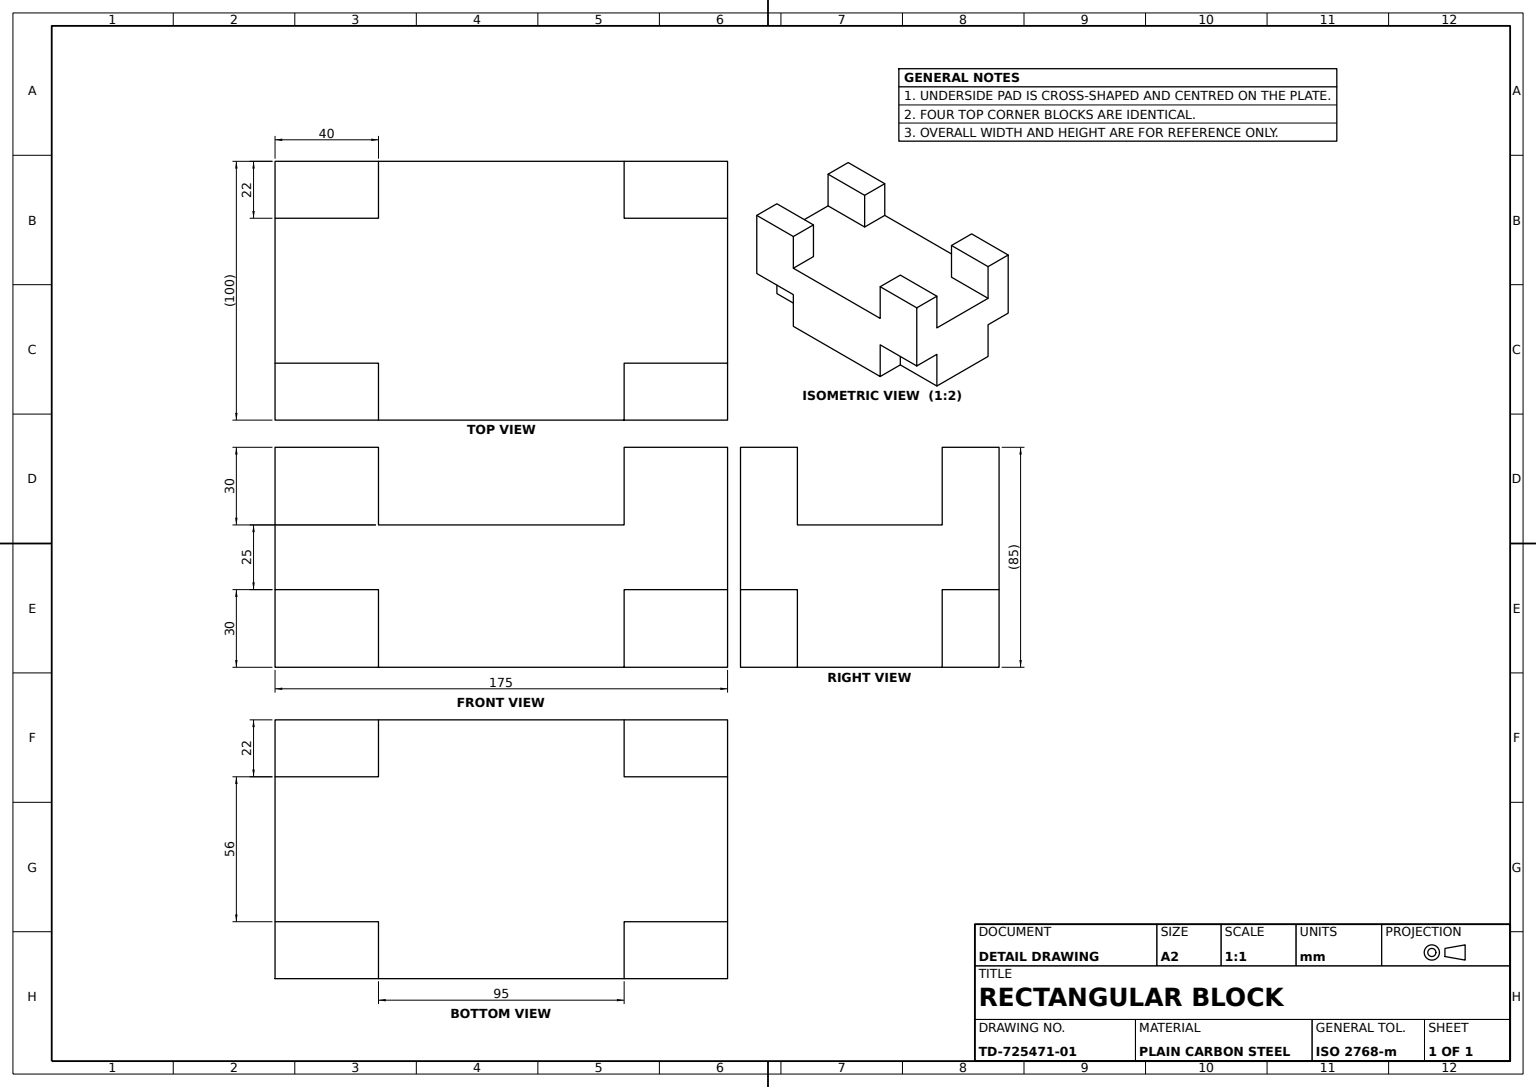
SolidWorks part; units mm, degrees
material "Plain Carbon Steel"
ref_plane "Front Plane" through (0, 0, 0) normal (0, 0, 1) x (1, 0, 0)
ref_plane "Top Plane" through (0, 0, 0) normal (0, 1, 0) x (1, 0, 0)
ref_plane "Right Plane" through (0, 0, 0) normal (1, 0, 0) x (0, 0, -1)
sketch "Base Plate Sketch" plane through (0, 0, 0) normal (0, 1, 0) x (1, 0, 0)
  line L1 (-87.5, -50) -> (87.5, -50)
  line L2 (-87.5, -50) -> (-87.5, 50)
  line L3 (-87.5, 50) -> (87.5, 50)
  line L4 (87.5, -50) -> (87.5, 50)
  point P0 (0, 0)
  dimension "D1" = 175
  dimension "D2" = 100
  dimension "D3" = 87.5
  dimension "D4" = 50
extrude "Base Plate 175x100x25" add sketch "Base Plate Sketch" along normal blind 25
sketch "Top Blocks Sketch" plane through (0, 25, 0) normal (0, 1, 0) x (1, 0, 0)
  line L1 (-87.5, -50) -> (-47.5, -50)
  line L2 (-87.5, -50) -> (-87.5, -28)
  line L3 (-87.5, -28) -> (-47.5, -28)
  line L4 (-47.5, -50) -> (-47.5, -28)
  line L5 (-87.5, 50) -> (-47.5, 50)
  line L6 (-87.5, 50) -> (-87.5, 28)
  line L7 (-87.5, 28) -> (-47.5, 28)
  line L8 (-47.5, 50) -> (-47.5, 28)
  line L9 (87.5, 50) -> (47.5, 50)
  line L10 (87.5, 50) -> (87.5, 28)
  line L11 (87.5, 28) -> (47.5, 28)
  line L12 (47.5, 50) -> (47.5, 28)
  line L13 (87.5, -50) -> (47.5, -50)
  line L14 (87.5, -50) -> (87.5, -28)
  line L15 (87.5, -28) -> (47.5, -28)
  line L16 (47.5, -50) -> (47.5, -28)
  dimension "D1" = 40
  dimension "D2" = 22
  dimension "D3" = 22
  dimension "D4" = 40
  dimension "D5" = 40
  dimension "D6" = 22
  dimension "D7" = 40
  dimension "D8" = 22
extrude "Top Blocks 4x40x22" add sketch "Top Blocks Sketch" along normal blind 30
sketch "Bottom Pads Sketch" plane through (0, 0, 0) normal (0, -1, 0) x (1, 0, 0)
  line L0 (-47.5, 50) -> (47.5, 50)
  line L3 (-87.5, -28) -> (-47.5, -28)
  line L4 (-47.5, -50) -> (-47.5, -28)
  line L7 (-87.5, 28) -> (-47.5, 28)
  line L8 (-47.5, 50) -> (-47.5, 28)
  line L11 (87.5, 28) -> (47.5, 28)
  line L12 (47.5, 50) -> (47.5, 28)
  line L15 (87.5, -28) -> (47.5, -28)
  line L16 (47.5, -50) -> (47.5, -28)
  line L17 (87.5, 28) -> (87.5, -28)
  line L18 (47.5, -50) -> (-47.5, -50)
  line L19 (-87.5, -28) -> (-87.5, 28)
  dimension "D1" = 22
  dimension "D2" = 95
  dimension "D3" = 40
  dimension "D4" = 56
  dimension "D5" = 40
  dimension "D6" = 87.5
  dimension "D7" = 40
  dimension "D8" = 50
extrude "Bottom Pads" add sketch "Bottom Pads Sketch" along normal blind 30
